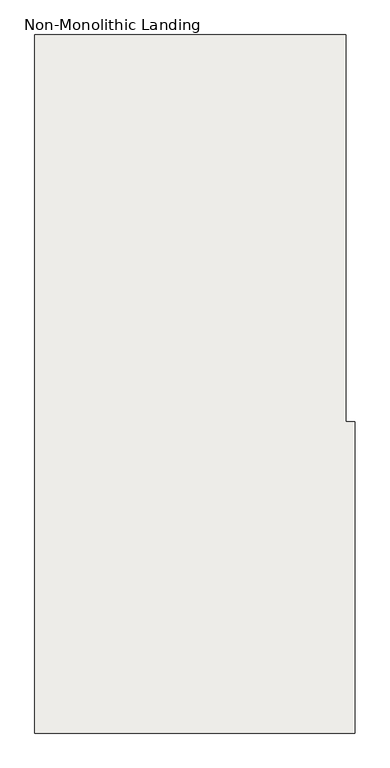
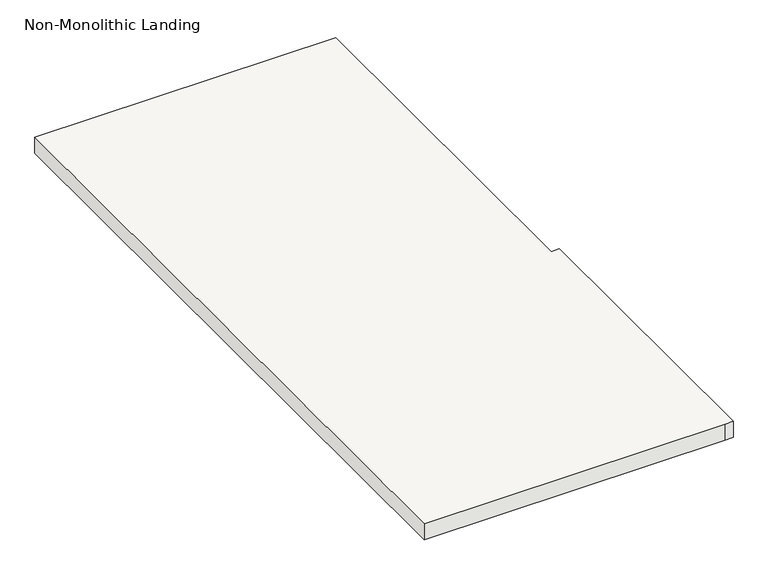
"""IFC4 building model written with IfcOpenShell, lengths in millimetres: slab geometry, Non-Monolithic Landing."""

from ifc_helpers import new_model, si_unit, origin, place, context, project, spatial, faceted_brep, source, transform, mapped, element, save


def non_monolithic_landing_64c69633(model_context):
    return source(origin(), model_context, "Body", "Brep", [
        faceted_brep([(-4484.3005972, 2819.495038, 1987.55), (-4458.9005972, 2819.495038, 2012.95), (-4458.9005972, 1905.095038, 2012.95), (-4484.3005972, 1905.095038, 1987.55), (-5373.3005972, 2819.495038, 2032.0), (-5373.3005972, 770.2870892, 2032.0), (-4458.9005972, 770.2870892, 2032.0), (-4433.5005972, 770.2870892, 2032.0), (-4433.5005972, 1684.6870892, 2032.0), (-4458.9005972, 1684.6870892, 2032.0), (-4458.9005972, 2819.495038, 2032.0), (-4484.3005972, 1905.095038, 1981.2), (-4458.9005972, 1905.095038, 1981.2), (-4458.9005972, 1684.6870892, 1981.2), (-4433.5005972, 1684.6870892, 1981.2), (-4433.5005972, 770.2870892, 1981.2), (-4458.9005972, 770.2870892, 1981.2), (-5373.3005972, 770.2870892, 1981.2), (-5373.3005972, 2819.495038, 1981.2), (-4484.3005972, 2819.495038, 1981.2)], [[[0, 1, 2, 3]], [[4, 5, 6, 7, 8, 9, 10]], [[11, 12, 13, 14, 15, 16, 17, 18, 19]], [[12, 11, 3, 2]], [[11, 19, 0, 3]], [[4, 10, 1, 0, 19, 18]], [[5, 4, 18, 17]], [[6, 5, 17, 16]], [[7, 6, 16, 15]], [[8, 7, 15, 14]], [[9, 8, 14, 13]], [[10, 9, 13, 12, 2, 1]]]),
    ])


if __name__ == "__main__":
    model = new_model("IFC4")
    model_context = context("Model", 3, world=origin())
    ifc_project = project(units=[si_unit("LENGTHUNIT", "METRE", prefix="MILLI")], contexts=[model_context])
    site = spatial("IfcSite", under=ifc_project)
    building = spatial("IfcBuilding", under=site)
    placement = place(None, origin())
    non_monolithic_landing_shape = non_monolithic_landing_64c69633(model_context)
    element("IfcSlab", 1, ObjectType="Non-Monolithic Landing", at=placement, inside=building, context=model_context, shape_type="MappedRepresentation", body=[
        mapped(non_monolithic_landing_shape, transform((0.0, 0.0, 0.0), x_axis=(1.0, 0.0, 0.0), y_axis=(0.0, 1.0, 0.0), z_axis=(0.0, 0.0, 1.0))),
    ])
    save(model, "model.ifc")

# Revit data of these elements
# Element 1 (IfcSlab, "Non-Monolithic Landing")
#   Materials on its faces: "Gypsum Wall Board"
# Materials
#   "Gypsum Wall Board": class "Generic", colour RGB 127 127 127, transparency 0, Description = "Gypsum Wall Board", Cost = 0
